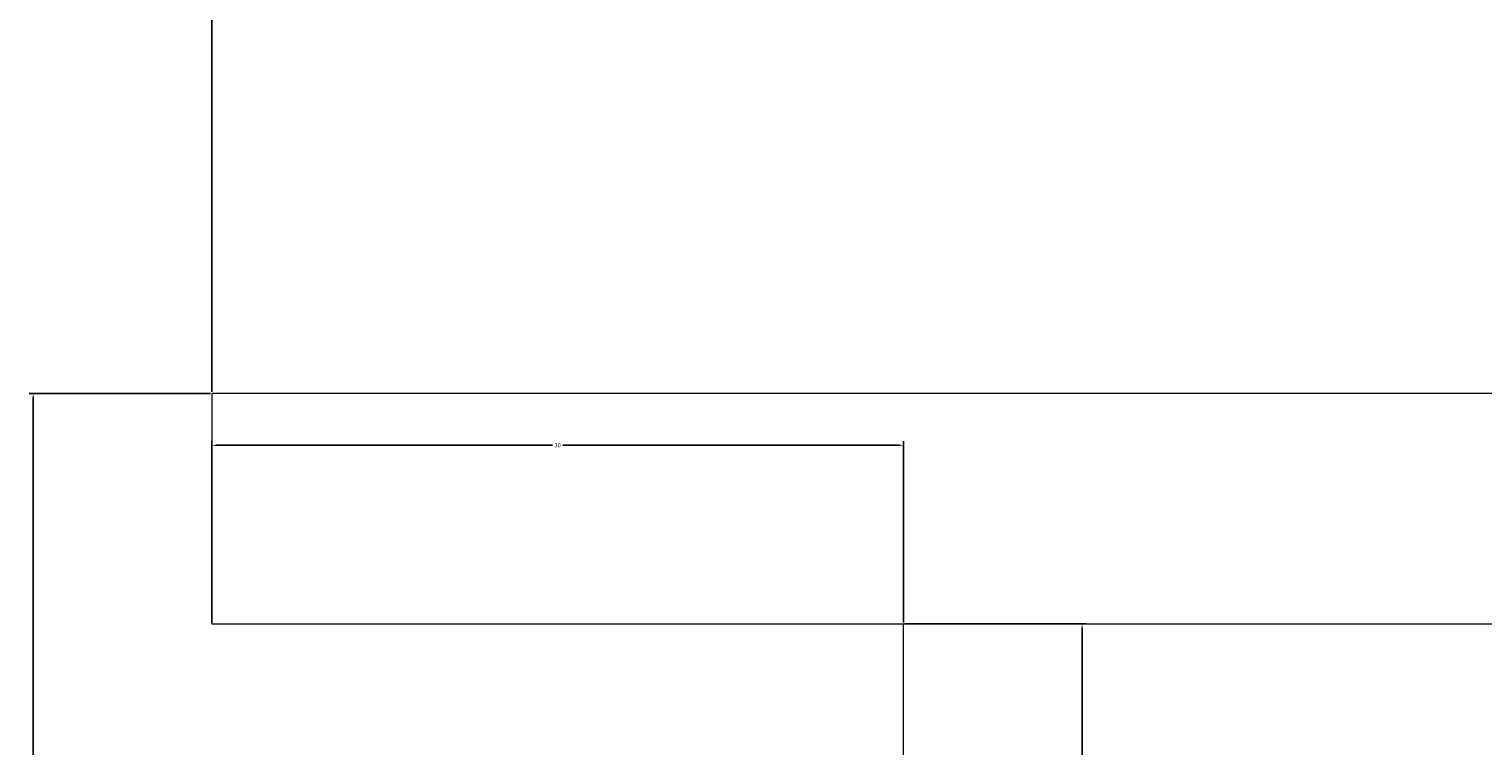
# Model space of a CAD drawing. Units: millimetres. Extents: x 118 to 244, y 285 to 440.
# Tile 2 of 4: x 118 to 181, y 331 to 362. Entities that reach past the tile are written whole.
import ezdxf

# ---------------------------------------------------------------- set-up
doc = ezdxf.new("R2010")
doc.units = ezdxf.units.MM
doc.layers.add('M-CONS', color=8, linetype='Continuous', lineweight=13)
doc.layers.add('M-DIMS', color=2, linetype='Continuous', lineweight=18)
doc.styles.get("Standard").update_dxf_attribs({"font": 'arial.ttf'})
doc.dimstyles.get("Standard").update_dxf_attribs({"dimtxt": 0.18, "dimasz": 0.18, "dimexe": 0.18, "dimexo": 0.0625, "dimgap": 0.09, "dimtad": 0, "dimtih": 1, "dimtoh": 1, "dimdec": 4, "dimzin": 0, "dimdsep": 46, "dimtxsty": 'Standard', "dimcen": 0.09, "dimadec": 0, "dimazin": 0, "dimtfac": 1, "dimtdec": 4, "dimtofl": 0, "dimtmove": 0, "dimatfit": 3, "dimfxl": 1, "dimtolj": 1, "dimtzin": 0, "dimarcsym": 0})

# ---------------------------------------------------------------- blocks, each defined once
blk = doc.blocks.new('*D2')
at = {"layer": 'Defpoints', "color": 0, "transparency": 16777216}
for p in [(117.774, 346.437), (125.524, 346.437), (125.524, 292.437)]:
    blk.add_point(p, dxfattribs=at)
at = {"layer": 'M-DIMS', "color": 0, "lineweight": -2, "transparency": 16777216}
for p, q in [((125.462, 346.437), (117.594, 346.437)), ((117.774, 346.257), (117.774, 319.618)), ((117.774, 292.617), (117.774, 319.255)), ((125.462, 292.437), (117.594, 292.437))]:
    blk.add_line(p, q, dxfattribs=at)
at = {"layer": 'M-DIMS', "color": 0, "transparency": 16777216}
for points in [[(117.744, 346.257), (117.804, 346.257), (117.774, 346.437)], [(117.744, 292.617), (117.804, 292.617), (117.774, 292.437)]]:
    blk.add_solid(points, dxfattribs=at)
at = {"layer": 'M-DIMS', "color": 0, "transparency": 16777216, "insert": (117.774, 319.437), "char_height": 0.18, "attachment_point": 5}
blk.add_mtext('\\A1;54', dxfattribs=at)
blk = doc.blocks.new('*D3')
at = {"layer": 'Defpoints', "color": 0, "transparency": 16777216}
for p in [(200.524, 439.795), (125.524, 346.437), (200.524, 346.437)]:
    blk.add_point(p, dxfattribs=at)
at = {"layer": 'M-DIMS', "color": 0, "lineweight": -2, "transparency": 16777216}
for p, q in [((125.524, 346.499), (125.524, 439.975)), ((125.704, 439.795), (162.805, 439.795)), ((200.344, 439.795), (163.243, 439.795)), ((200.524, 346.499), (200.524, 439.975))]:
    blk.add_line(p, q, dxfattribs=at)
at = {"layer": 'M-DIMS', "color": 0, "transparency": 16777216}
for points in [[(125.704, 439.825), (125.704, 439.765), (125.524, 439.795)], [(200.344, 439.825), (200.344, 439.765), (200.524, 439.795)]]:
    blk.add_solid(points, dxfattribs=at)
at = {"layer": 'M-DIMS', "color": 0, "transparency": 16777216, "insert": (163.024, 439.795), "char_height": 0.18, "attachment_point": 5}
blk.add_mtext('\\A1;75', dxfattribs=at)
blk = doc.blocks.new('*D6')
at = {"layer": 'Defpoints', "color": 0, "transparency": 16777216}
for p in [(155.524, 336.437), (155.524, 322.437), (163.274, 322.437)]:
    blk.add_point(p, dxfattribs=at)
at = {"layer": 'M-DIMS', "color": 0, "lineweight": -2, "transparency": 16777216}
for p, q in [((155.587, 336.437), (163.454, 336.437)), ((163.274, 336.257), (163.274, 329.617)), ((163.274, 322.617), (163.274, 329.257)), ((155.587, 322.437), (163.454, 322.437))]:
    blk.add_line(p, q, dxfattribs=at)
at = {"layer": 'M-DIMS', "color": 0, "transparency": 16777216}
for points in [[(163.244, 336.257), (163.304, 336.257), (163.274, 336.437)], [(163.244, 322.617), (163.304, 322.617), (163.274, 322.437)]]:
    blk.add_solid(points, dxfattribs=at)
at = {"layer": 'M-DIMS', "color": 0, "transparency": 16777216, "insert": (163.274, 329.437), "char_height": 0.18, "attachment_point": 5}
blk.add_mtext('\\A1;14', dxfattribs=at)
blk = doc.blocks.new('*D9')
at = {"layer": 'Defpoints', "color": 0, "transparency": 16777216}
for p in [(235.677, 439.795), (235.677, 432.045), (125.524, 346.437)]:
    blk.add_point(p, dxfattribs=at)
at = {"layer": 'M-DIMS', "color": 0, "lineweight": -2, "transparency": 16777216}
for p, q in [((125.524, 346.499), (125.524, 439.975)), ((125.704, 439.795), (180.145, 439.795)), ((235.497, 439.795), (181.056, 439.795)), ((235.677, 432.107), (235.677, 439.975))]:
    blk.add_line(p, q, dxfattribs=at)
at = {"layer": 'M-DIMS', "color": 0, "transparency": 16777216}
for points in [[(125.704, 439.825), (125.704, 439.765), (125.524, 439.795)], [(235.497, 439.825), (235.497, 439.765), (235.677, 439.795)]]:
    blk.add_solid(points, dxfattribs=at)
at = {"layer": 'M-DIMS', "color": 0, "transparency": 16777216, "insert": (180.6, 439.795), "char_height": 0.18, "attachment_point": 5}
blk.add_mtext('\\A1;110.15', dxfattribs=at)
blk = doc.blocks.new('*D10')
at = {"layer": 'Defpoints', "color": 0, "transparency": 16777216}
for p in [(235.677, 432.045), (243.427, 432.045), (125.524, 292.437)]:
    blk.add_point(p, dxfattribs=at)
at = {"layer": 'M-DIMS', "color": 0, "lineweight": -2, "transparency": 16777216}
for p, q in [((235.739, 432.045), (243.607, 432.045)), ((243.427, 431.865), (243.427, 362.423)), ((243.427, 292.617), (243.427, 362.059)), ((125.587, 292.437), (243.607, 292.437))]:
    blk.add_line(p, q, dxfattribs=at)
at = {"layer": 'M-DIMS', "color": 0, "transparency": 16777216}
for points in [[(243.397, 431.865), (243.457, 431.865), (243.427, 432.045)], [(243.397, 292.617), (243.457, 292.617), (243.427, 292.437)]]:
    blk.add_solid(points, dxfattribs=at)
at = {"layer": 'M-DIMS', "color": 0, "transparency": 16777216, "insert": (243.427, 362.241), "char_height": 0.18, "attachment_point": 5}
blk.add_mtext('\\A1;139.6', dxfattribs=at)
blk = doc.blocks.new('*D11')
at = {"layer": 'Defpoints', "color": 0, "transparency": 16777216}
for p in [(155.524, 344.187), (125.524, 336.437), (155.524, 336.437)]:
    blk.add_point(p, dxfattribs=at)
at = {"layer": 'M-DIMS', "color": 0, "lineweight": -2, "transparency": 16777216}
for p, q in [((125.524, 336.499), (125.524, 344.367)), ((155.524, 336.499), (155.524, 344.367)), ((125.704, 344.187), (140.306, 344.187)), ((155.344, 344.187), (140.743, 344.187))]:
    blk.add_line(p, q, dxfattribs=at)
at = {"layer": 'M-DIMS', "color": 0, "transparency": 16777216}
for points in [[(125.704, 344.217), (125.704, 344.157), (125.524, 344.187)], [(155.344, 344.217), (155.344, 344.157), (155.524, 344.187)]]:
    blk.add_solid(points, dxfattribs=at)
at = {"layer": 'M-DIMS', "color": 0, "transparency": 16777216, "insert": (140.524, 344.187), "char_height": 0.18, "attachment_point": 5}
blk.add_mtext('\\A1;30', dxfattribs=at)

msp = doc.modelspace()

# ---------------------------------------------------------------- linework, layer by layer
at = {"layer": 'M-CONS'}
for p, q in [((150.5241, 336.4369, 20), (210.5241, 336.4369, 20)), ((155.5241, 322.4369, 10), (155.5241, 336.4369, 10))]:
    msp.add_line(p, q, dxfattribs=at)
at = {"layer": 'M-CONS', "elevation": 10}
msp.add_lwpolyline([(125.5241, 336.4369), (155.5241, 336.4369), (200.5241, 336.4369), (200.5241, 346.4369), (125.5241, 346.4369)], close=True, dxfattribs=at)
at = {"layer": 'M-CONS', "extrusion": (0, -1, 0)}
msp.add_arc((150.5241, 45, -336.4369), 25, 180, 270, dxfattribs=at)

# ---------------------------------------------------------------- dimensions: what is measured, and where the dimension line sits
at = {"layer": 'M-DIMS'}
for base, p1, p2, override, picture, middle in [((200.5241, 439.7945), (125.5241, 346.4369), (200.5241, 346.4369), {"dimdec": 0, "dimlfac": 1, "dimrnd": 0, "dimzin": 0, "dimdsep": 46, "dimlunit": 2}, '*D3', (163.0241, 439.7945)), ((235.6768, 439.7945), (125.5241, 346.4369), (235.6768, 432.0445), {"dimdec": 2, "dimlfac": 1, "dimrnd": 0, "dimzin": 0, "dimdsep": 46, "dimlunit": 2}, '*D9', (180.6005, 439.7945)), ((155.5241, 344.1869), (125.5241, 336.4369), (155.5241, 336.4369), {"dimdec": 0, "dimlfac": 1, "dimrnd": 0, "dimzin": 0, "dimdsep": 46, "dimlunit": 2}, '*D11', (140.5241, 344.1869))]:
    dim = msp.add_linear_dim(base=base, p1=p1, p2=p2, dimstyle='Standard', override=override, dxfattribs=at)
    dim.commit()
    dim.dimension.update_dxf_attribs({"geometry": picture, "text_midpoint": middle})
for base, p1, p2, angle, override, picture, middle in [((243.4268, 432.0445), (125.5241, 292.4369), (235.6768, 432.0445), 90, {"dimdec": 1, "dimlfac": 1, "dimrnd": 0, "dimzin": 0, "dimdsep": 46, "dimlunit": 2}, '*D10', (243.4268, 362.2407)), ((117.7741, 346.4369), (125.5241, 292.4369), (125.5241, 346.4369), 90, {"dimdec": 0, "dimlfac": 1, "dimrnd": 0, "dimzin": 0, "dimdsep": 46, "dimlunit": 2}, '*D2', (117.7741, 319.4369)), ((163.2741, 322.4369), (155.5241, 336.4369), (155.5241, 322.4369), 270, {"dimdec": 0, "dimlfac": 1, "dimrnd": 0, "dimzin": 0, "dimdsep": 46, "dimlunit": 2}, '*D6', (163.2741, 329.4369))]:
    dim = msp.add_linear_dim(base=base, p1=p1, p2=p2, angle=angle, dimstyle='Standard', override=override, dxfattribs=at)
    dim.commit()
    dim.dimension.update_dxf_attribs({"geometry": picture, "text_midpoint": middle})

doc.saveas('drawing.dxf')
